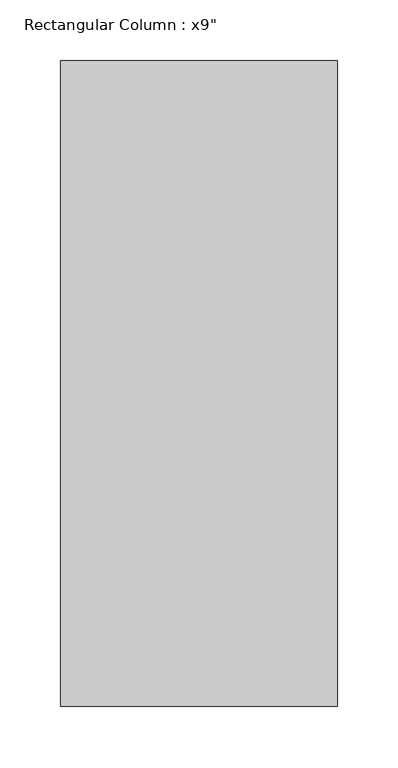
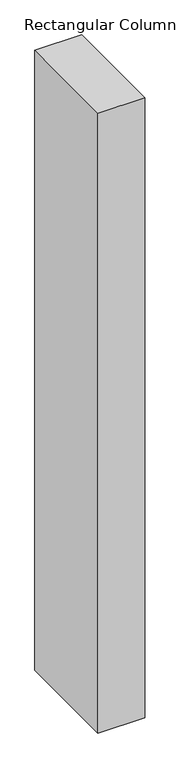
"""IFC4 building model written with IfcOpenShell, lengths in millimetres: column geometry."""

from ifc_helpers import new_model, si_unit, origin, origin_with_axes, place, context, project, spatial, polyline, outline, extrude, source, transform, mapped, element, save


def column_1de33f28(model_context):
    return source(origin(), model_context, "Body", "SweptSolid", [
        extrude(outline(polyline([(114.3, 266.7), (114.3, -266.7), (-114.3, -266.7), (-114.3, 266.7), (114.3, 266.7)])), origin_with_axes(), (0.0, 0.0, 1.0), 3200.4),
    ])


if __name__ == "__main__":
    model = new_model("IFC4")
    model_context = context("Model", 3, world=origin())
    ifc_project = project(units=[si_unit("LENGTHUNIT", "METRE", prefix="MILLI")], contexts=[model_context])
    site = spatial("IfcSite", under=ifc_project)
    building = spatial("IfcBuilding", under=site)
    placement = place(None, origin())
    column_shape = column_1de33f28(model_context)
    element("IfcColumn", 1, ObjectType="Rectangular Column : x9\"", at=placement, inside=building, context=model_context, shape_type="MappedRepresentation", body=[
        mapped(column_shape, transform((0.0, 0.0, 0.0), x_axis=(1.0, 0.0, 0.0), y_axis=(0.0, 1.0, 0.0), z_axis=(0.0, 0.0, 1.0))),
    ])
    save(model, "model.ifc")

# Revit data of these elements
# Type "Rectangular Column : x9\""
#   Assembly Code = "B1010200"
#   Depth = 1' - 9"
#   Offset Base = 0' - 0"
#   Offset Top = 0' - 0"
#   Width = 0' - 9"
#   Material = none
